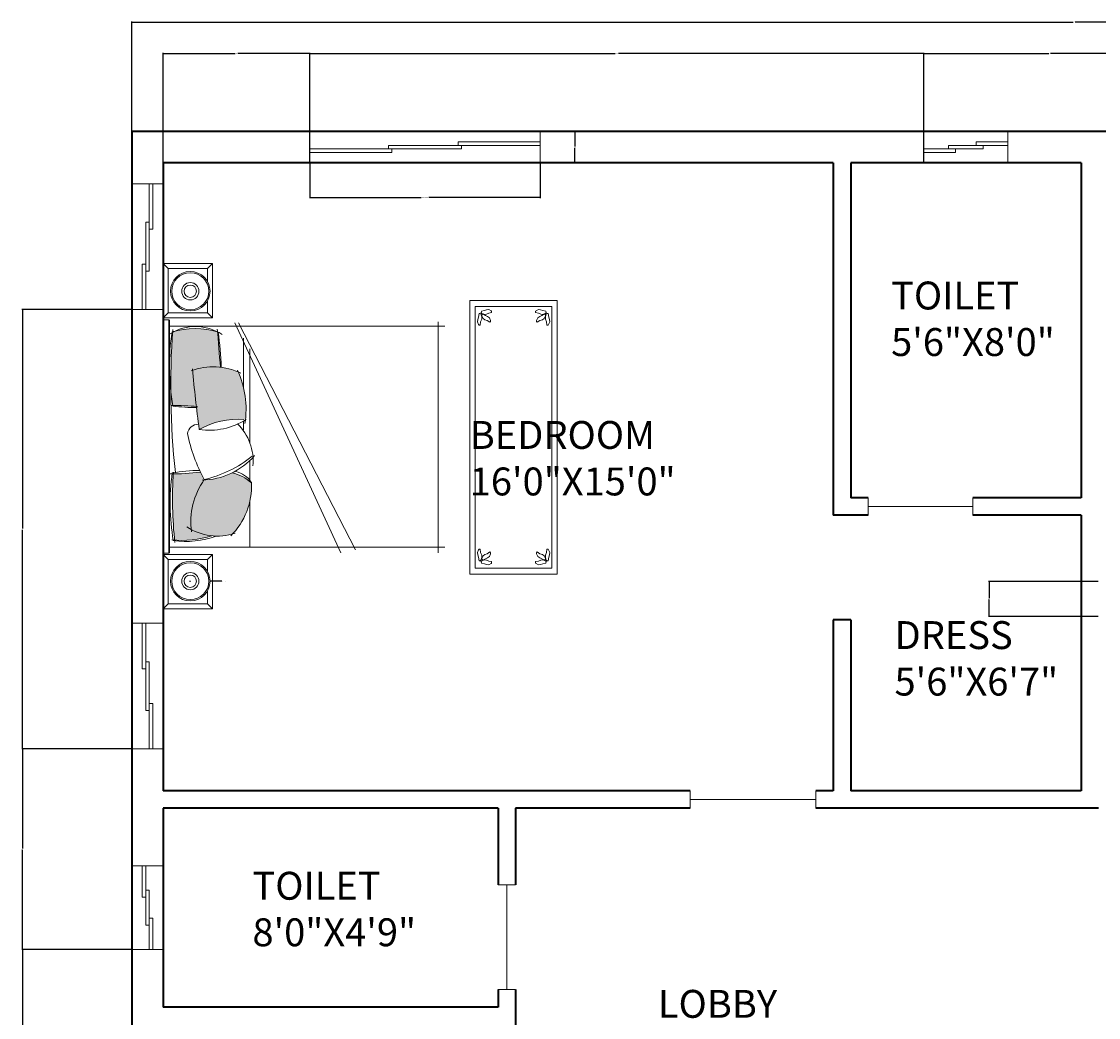
# Model space of a CAD drawing. Units: inches. Extents: x 1569 to 2779, y 1228 to 1844.
# Tile 3 of 6: x 1569 to 1878, y 1559 to 1844. Entities that reach past the tile are written whole.
import ezdxf

# ---------------------------------------------------------------- set-up
doc = ezdxf.new("R2010")
doc.units = ezdxf.units.IN
for name, color, linetype, lineweight in [('0.10', 252, 'Continuous', 9), ('0.15', 34, 'Continuous', 15), ('A-ANNO-DIMS', 2, 'Continuous', 18), ('A-AREA-IDEN', 7, 'Continuous', 18), ('A-DOOR', 3, 'Continuous', 20), ('A-FURN', 8, 'Continuous', 13), ('A-FURN-PATT', 116, 'Continuous', 9), ('A-GLAZ', 5, 'Continuous', 18), ('A-WALL', 7, 'Continuous', 35)]:
    doc.layers.add(name, color=color, linetype=linetype, lineweight=lineweight)
doc.styles.get("Standard").update_dxf_attribs({"font": 'arial.ttf'})
doc.dimstyles.get("Standard").update_dxf_attribs({"dimtxt": 0.18, "dimasz": 0.18, "dimexe": 0.18, "dimexo": 0.0625, "dimgap": 0.09, "dimtad": 0, "dimtih": 1, "dimtoh": 1, "dimdec": 4, "dimzin": 0, "dimdsep": 46, "dimtxsty": 'Standard', "dimcen": 0.09, "dimadec": 0, "dimazin": 0, "dimtfac": 1, "dimtdec": 4, "dimtofl": 0, "dimtmove": 0, "dimatfit": 3, "dimfxl": 1, "dimtolj": 1, "dimtzin": 0, "dimarcsym": 0})

# ---------------------------------------------------------------- blocks, each defined once
blk = doc.blocks.new('camita')
at = {"layer": '0.10'}
for p, q in [((-0.85, -0.045), (0.85, -0.045)), ((-0.805, -0.045), (-0.805, -2.0485)), ((0.805, -0.045), (0.805, -2.0485)), ((-0.8271, -0.521), (0.8464, -1.2932)), ((-0.8271, -0.5476), (0.8236, -1.3992)), ((-0.7161, -0.585), (-0.3554, -0.585)), ((-0.1136, -0.585), (-0.0485, -0.585)), ((-0.638, -0.63), (0.0434, -0.63)), ((0.1749, -0.63), (0.3179, -0.63)), ((0.4739, -0.63), (0.805, -0.63)), ((-0.8354, -2), (0.8464, -2))]:
    blk.add_line(p, q, dxfattribs=at)
blk.add_lwpolyline([(-0.85, -0.0405), (0.85, -0.0405), (0.85, 0), (-0.85, 0)], close=True, dxfattribs=at)
for centre, radius, start, end in [((-0.4574, -0.2364), 0.3443, 147.50996, 213.83359), ((-0.1997, -0.2266), 0.5864, 163.92635, 197.14087), ((-0.3639, -5.8457), 5.7909, 83.80731, 94.12107), ((-0.5104, -1.7232), 1.6781, 80.12554, 98.66187), ((2.3534, -0.0532), 2.5803, 180.10628, 184.38541), ((-1.5443, -0.2452), 1.3333, 359.93941, 7.55329), ((1.5815, -0.2893), 1.3353, 170.38021, 178.99138), ((-1.4396, -0.0609), 1.7117, 352.92911, 0.39592), ((0.4524, -3.0675), 2.9996, 83.90257, 93.67595), ((0.4863, -1.6286), 1.5781, 80.16015, 98.05996), ((0.0294, -0.1377), 0.7262, 342.58415, 6.00484), ((0.1326, -0.1696), 0.6307, 339.92303, 8.74334), ((-0.0543, -0.3633), 0.4542, 159.30257, 206.50263), ((-1.3301, -9.6748), 9.4985, 82.27078, 84.93989), ((-0.007, -0.258), 0.0828, 100.01798, 179.73597), ((-0.2931, -1.4378), 1.2903, 61.97485, 77.84351), ((0.6265, -0.7518), 0.5508, 82.96906, 124.67388), ((0.3203, -0.3944), 0.4043, 341.45245, 33.45121), ((0.4585, -0.5454), 0.5842, 151.04555, 184.14969), ((-0.5341, -0.3393), 0.4875, 327.26442, 9.0473), ((-0.1986, -0.2742), 0.5159, 310.73945, 359.05759), ((-0.5673, -0.0868), 0.9057, 321.69527, 346.46261), ((-1.8672, -14.986), 14.6323, 84.65974, 85.75157), ((-0.4598, 1.4861), 1.9092, 260.95299, 268.65169), ((-0.2002, 0.064), 0.6673, 244.78094, 279.06058), ((0.179, -0.272), 0.3828, 224.52836, 275.22287), ((0.4384, -0.4834), 0.1898, 193.68485, 236.70352), ((0.5707, -0.4317), 0.3145, 192.93877, 221.96363), ((0.3612, -0.133), 0.5096, 267.25889, 315.29965)]:
    blk.add_arc(centre, radius, start, end, dxfattribs=at)
blk = doc.blocks.new('VELADOR')
at = {"layer": '0.15'}
for p, q in [((-0.2475, 0), (-0.2025, -0.045)), ((0.2475, 0), (0.2025, -0.045)), ((-0.2025, -0.405), (-0.2475, -0.45)), ((0.2475, -0.45), (0.2025, -0.405))]:
    blk.add_line(p, q, dxfattribs=at)
blk.add_lwpolyline([(-0.2475, 0), (-0.2475, -0.45), (0.2475, -0.45), (0.2475, 0)], close=True, dxfattribs=at)
blk.add_lwpolyline([(0.0921, -0.405), (0.2025, -0.405), (0.2025, -0.045), (-0.2025, -0.045), (-0.2025, -0.405), (-0.0818, -0.405)], dxfattribs=at)
for radius in [0.18, 0.1688, 0.0788, 0.0563]:
    blk.add_circle((0.0052, -0.2474), radius, dxfattribs=at)
blk = doc.blocks.new('carpet-7')
at = {"color": 0, "linetype": 'ByBlock'}
for p, q in [((-1.0224, 0), (0, 0)), ((0, 0), (0, -0.54)), ((-1.694, -0.54), (-1.694, 0)), ((-1.694, 0), (-1.0224, 0)), ((-1.658, -0.5076), (-1.658, -0.0324)), ((-1.658, -0.0324), (-0.036, -0.0324)), ((-1.6112, -0.0562), (-1.6124, -0.0637)), ((-1.6124, -0.0637), (-1.6088, -0.068)), ((-1.5896, -0.0518), (-1.6112, -0.0562)), ((-1.5752, -0.0486), (-1.5896, -0.0518)), ((-1.5764, -0.0724), (-1.5608, -0.0659)), ((-1.5608, -0.0464), (-1.5752, -0.0486)), ((-1.544, -0.0529), (-1.5608, -0.0464)), ((-1.5608, -0.0659), (-1.5404, -0.0637)), ((-1.5404, -0.0562), (-1.544, -0.0529)), ((-1.5404, -0.0637), (-1.5404, -0.0562)), ((-0.1512, -0.0562), (-0.1476, -0.0529)), ((-0.1512, -0.0637), (-0.1512, -0.0562)), ((-0.1308, -0.0659), (-0.1512, -0.0637)), ((-0.1476, -0.0529), (-0.1308, -0.0464)), ((-0.1308, -0.0464), (-0.1164, -0.0486)), ((-0.1152, -0.0724), (-0.1308, -0.0659)), ((-0.1164, -0.0486), (-0.102, -0.0518)), ((-0.102, -0.0518), (-0.0804, -0.0562)), ((-0.0792, -0.0637), (-0.0828, -0.068)), ((-0.0804, -0.0562), (-0.0792, -0.0637)), ((-0.036, -0.0324), (-0.036, -0.5076)), ((-1.6364, -0.1156), (-1.634, -0.1026)), ((-1.6292, -0.1307), (-1.6364, -0.1156)), ((-1.634, -0.1026), (-1.6304, -0.0896)), ((-1.6304, -0.0896), (-1.6256, -0.0702)), ((-1.6256, -0.1339), (-1.6292, -0.1307)), ((-1.6256, -0.0702), (-1.6172, -0.0691)), ((-1.6172, -0.0691), (-1.6124, -0.0724)), ((-1.6148, -0.1156), (-1.6172, -0.1339)), ((-1.6076, -0.1015), (-1.6148, -0.1156)), ((-1.6124, -0.0724), (-1.6064, -0.0886)), ((-1.6088, -0.068), (-1.5908, -0.0734)), ((-1.6088, -0.0788), (-1.6028, -0.0724)), ((-1.5992, -0.0961), (-1.6088, -0.0788)), ((-1.6064, -0.0886), (-1.6076, -0.1015)), ((-1.6028, -0.0724), (-1.5968, -0.0724)), ((-1.5932, -0.108), (-1.5992, -0.0961)), ((-1.5968, -0.0724), (-1.5812, -0.081)), ((-1.5848, -0.1199), (-1.5932, -0.108)), ((-1.5908, -0.0734), (-1.5764, -0.0724)), ((-1.5692, -0.1274), (-1.5848, -0.1199)), ((-1.5812, -0.081), (-1.5728, -0.0918)), ((-1.5728, -0.0918), (-1.568, -0.1069)), ((-1.5632, -0.1274), (-1.5692, -0.1274)), ((-1.568, -0.1069), (-1.5572, -0.1231)), ((-1.5572, -0.1231), (-1.5632, -0.1274)), ((-0.1236, -0.1069), (-0.1344, -0.1231)), ((-0.1344, -0.1231), (-0.1284, -0.1274)), ((-0.1284, -0.1274), (-0.1224, -0.1274)), ((-0.1188, -0.0918), (-0.1236, -0.1069)), ((-0.1224, -0.1274), (-0.1068, -0.1199)), ((-0.1104, -0.081), (-0.1188, -0.0918)), ((-0.1008, -0.0734), (-0.1152, -0.0724)), ((-0.0948, -0.0724), (-0.1104, -0.081)), ((-0.1068, -0.1199), (-0.0984, -0.108)), ((-0.0828, -0.068), (-0.1008, -0.0734)), ((-0.0984, -0.108), (-0.0924, -0.0961)), ((-0.0888, -0.0724), (-0.0948, -0.0724)), ((-0.0924, -0.0961), (-0.0828, -0.0788)), ((-0.0828, -0.0788), (-0.0888, -0.0724)), ((-0.0792, -0.0724), (-0.0852, -0.0886)), ((-0.0852, -0.0886), (-0.084, -0.1015)), ((-0.084, -0.1015), (-0.0768, -0.1156)), ((-0.0744, -0.0691), (-0.0792, -0.0724)), ((-0.0768, -0.1156), (-0.0744, -0.1339)), ((-0.066, -0.0702), (-0.0744, -0.0691)), ((-0.0612, -0.0896), (-0.066, -0.0702)), ((-0.066, -0.1339), (-0.0624, -0.1307)), ((-0.0624, -0.1307), (-0.0552, -0.1156)), ((-0.0576, -0.1026), (-0.0612, -0.0896)), ((-0.0552, -0.1156), (-0.0576, -0.1026)), ((-1.6172, -0.1339), (-1.6256, -0.1339)), ((-0.0744, -0.1339), (-0.066, -0.1339)), ((-1.6292, -0.4093), (-1.6364, -0.4244)), ((-1.6364, -0.4244), (-1.634, -0.4374)), ((-1.634, -0.4374), (-1.6304, -0.4504)), ((-1.6304, -0.4504), (-1.6256, -0.4698)), ((-1.6256, -0.4061), (-1.6292, -0.4093)), ((-1.6172, -0.4061), (-1.6256, -0.4061)), ((-1.6148, -0.4244), (-1.6172, -0.4061)), ((-1.6076, -0.4385), (-1.6148, -0.4244)), ((-1.6124, -0.4676), (-1.6064, -0.4514)), ((-1.5992, -0.4439), (-1.6088, -0.4612)), ((-1.6088, -0.4612), (-1.6028, -0.4676)), ((-1.6088, -0.472), (-1.5908, -0.4666)), ((-1.6064, -0.4514), (-1.6076, -0.4385)), ((-1.5932, -0.432), (-1.5992, -0.4439)), ((-1.5968, -0.4676), (-1.5812, -0.459)), ((-1.5848, -0.4201), (-1.5932, -0.432)), ((-1.5908, -0.4666), (-1.5764, -0.4676)), ((-1.5692, -0.4126), (-1.5848, -0.4201)), ((-1.5812, -0.459), (-1.5728, -0.4482)), ((-1.5728, -0.4482), (-1.568, -0.4331)), ((-1.5632, -0.4126), (-1.5692, -0.4126)), ((-1.568, -0.4331), (-1.5572, -0.4169)), ((-1.5572, -0.4169), (-1.5632, -0.4126)), ((-0.1344, -0.4169), (-0.1284, -0.4126)), ((-0.1236, -0.4331), (-0.1344, -0.4169)), ((-0.1284, -0.4126), (-0.1224, -0.4126)), ((-0.1188, -0.4482), (-0.1236, -0.4331)), ((-0.1224, -0.4126), (-0.1068, -0.4201)), ((-0.1104, -0.459), (-0.1188, -0.4482)), ((-0.1008, -0.4666), (-0.1152, -0.4676)), ((-0.0948, -0.4676), (-0.1104, -0.459)), ((-0.1068, -0.4201), (-0.0984, -0.432)), ((-0.0828, -0.472), (-0.1008, -0.4666)), ((-0.0984, -0.432), (-0.0924, -0.4439)), ((-0.0924, -0.4439), (-0.0828, -0.4612)), ((-0.0828, -0.4612), (-0.0888, -0.4676)), ((-0.0852, -0.4514), (-0.084, -0.4385)), ((-0.0792, -0.4676), (-0.0852, -0.4514)), ((-0.084, -0.4385), (-0.0768, -0.4244)), ((-0.0768, -0.4244), (-0.0744, -0.4061)), ((-0.0744, -0.4061), (-0.066, -0.4061)), ((-0.066, -0.4061), (-0.0624, -0.4093)), ((-0.0612, -0.4504), (-0.066, -0.4698)), ((-0.0624, -0.4093), (-0.0552, -0.4244)), ((-0.0576, -0.4374), (-0.0612, -0.4504)), ((-0.0552, -0.4244), (-0.0576, -0.4374)), ((-1.658, -0.5076), (-0.036, -0.5076)), ((-1.6256, -0.4698), (-1.6172, -0.4709)), ((-1.6172, -0.4709), (-1.6124, -0.4676)), ((-1.6124, -0.4763), (-1.6088, -0.472)), ((-1.6112, -0.4838), (-1.6124, -0.4763)), ((-1.5896, -0.4882), (-1.6112, -0.4838)), ((-1.6028, -0.4676), (-1.5968, -0.4676)), ((-1.5752, -0.4914), (-1.5896, -0.4882)), ((-1.5764, -0.4676), (-1.5608, -0.4741)), ((-1.5608, -0.4936), (-1.5752, -0.4914)), ((-1.5608, -0.4741), (-1.5404, -0.4763)), ((-1.544, -0.4871), (-1.5608, -0.4936)), ((-1.5404, -0.4838), (-1.544, -0.4871)), ((-1.5404, -0.4763), (-1.5404, -0.4838)), ((-0.1308, -0.4741), (-0.1512, -0.4763)), ((-0.1512, -0.4763), (-0.1512, -0.4838)), ((-0.1512, -0.4838), (-0.1476, -0.4871)), ((-0.1476, -0.4871), (-0.1308, -0.4936)), ((-0.1152, -0.4676), (-0.1308, -0.4741)), ((-0.1308, -0.4936), (-0.1164, -0.4914)), ((-0.1164, -0.4914), (-0.102, -0.4882)), ((-0.102, -0.4882), (-0.0804, -0.4838)), ((-0.0888, -0.4676), (-0.0948, -0.4676)), ((-0.0792, -0.4763), (-0.0828, -0.472)), ((-0.0804, -0.4838), (-0.0792, -0.4763)), ((-0.0744, -0.4709), (-0.0792, -0.4676)), ((-0.066, -0.4698), (-0.0744, -0.4709)), ((0, -0.54), (-1.694, -0.54))]:
    blk.add_line(p, q, dxfattribs=at)
blk = doc.blocks.new('WIN-24IN')
for p, q in [((9, 24), (0, 24)), ((3, 24), (3, 15)), ((4, 24), (4, 7)), ((4, 17), (5, 17)), ((5, 17), (5, 0)), ((3, 15), (4, 15)), ((4, 7), (5, 7)), ((5, 9), (6, 9)), ((6, 9), (6, 0)), ((9, 0), (0, 0))]:
    blk.add_line(p, q)
blk = doc.blocks.new('WIN-66IN')
for p, q in [((0, 0), (0, 9)), ((66, 0), (66, 9)), ((0, 4), (43.5, 4)), ((22.5, 5), (66, 5)), ((22.5, 4), (22.5, 5)), ((23.5, 3), (23.5, 4)), ((42.5, 6), (66, 6)), ((42.5, 5), (42.5, 6)), ((43.5, 4), (43.5, 5)), ((0, 3), (23.5, 3))]:
    blk.add_line(p, q)
blk = doc.blocks.new('WIN-36IN-B')
for p, q in [((0, 36), (9, 36)), ((3, 23), (3, 36)), ((4, 11), (4, 36)), ((5, 25), (4, 25)), ((5, 0), (5, 25)), ((4, 23), (3, 23)), ((6, 13), (5, 13)), ((6, 0), (6, 13)), ((5, 11), (4, 11)), ((0, 0), (9, 0))]:
    blk.add_line(p, q)
blk = doc.blocks.new('DOOR-30IN')
for p, q in [((0, 5), (0, 0)), ((30, 5), (30, 0)), ((0, 2.5), (30, 2.5))]:
    blk.add_line(p, q)
blk = doc.blocks.new('DOOR-36IN')
for p, q in [((0, 5), (0, 0)), ((36, 5), (36, 0)), ((36, 2.5), (0, 2.5))]:
    blk.add_line(p, q)
blk = doc.blocks.new('*D29')
at = {"layer": 'A-ANNO-DIMS', "color": 0, "lineweight": -2, "transparency": 16777216}
for p, q in [((1652.06, 1803.82), (1652.06, 1793.8)), ((1718.06, 1803.82), (1718.06, 1793.8)), ((1652.24, 1793.98), (1683.94, 1793.98)), ((1717.88, 1793.98), (1686.18, 1793.98))]:
    blk.add_line(p, q, dxfattribs=at)
at = {"layer": 'A-ANNO-DIMS', "color": 0, "transparency": 16777216}
for points in [[(1652.24, 1794.01), (1652.24, 1793.95), (1652.06, 1793.98)], [(1717.88, 1794.01), (1717.88, 1793.95), (1718.06, 1793.98)]]:
    blk.add_solid(points, dxfattribs=at)
at = {"layer": 'Defpoints', "color": 0, "transparency": 16777216}
for p in [(1652.06, 1803.88), (1718.06, 1803.88), (1718.06, 1793.98)]:
    blk.add_point(p, dxfattribs=at)
at = {"layer": 'A-ANNO-DIMS', "color": 0, "transparency": 16777216, "insert": (1685.06, 1793.98), "char_height": 0.18, "attachment_point": 5}
blk.add_mtext('\\A1;WINDOW 66 TYP.', dxfattribs=at)
blk = doc.blocks.new('*D30')
at = {"layer": 'A-ANNO-DIMS', "color": 0, "lineweight": -2, "transparency": 16777216}
for p, q in [((1718.12, 1812.88), (1728.14, 1812.88)), ((1727.96, 1812.7), (1727.96, 1808.56)), ((1727.96, 1804.06), (1727.96, 1808.2)), ((1718.12, 1803.88), (1728.14, 1803.88))]:
    blk.add_line(p, q, dxfattribs=at)
at = {"layer": 'A-ANNO-DIMS', "color": 0, "transparency": 16777216}
for points in [[(1727.93, 1812.7), (1727.99, 1812.7), (1727.96, 1812.88)], [(1727.93, 1804.06), (1727.99, 1804.06), (1727.96, 1803.88)]]:
    blk.add_solid(points, dxfattribs=at)
at = {"layer": 'Defpoints', "color": 0, "transparency": 16777216}
for p in [(1718.06, 1812.88), (1727.96, 1812.88), (1718.06, 1803.88)]:
    blk.add_point(p, dxfattribs=at)
at = {"layer": 'A-ANNO-DIMS', "color": 0, "transparency": 16777216, "insert": (1727.96, 1808.38), "char_height": 0.18, "attachment_point": 5}
blk.add_mtext('\\A1;9 TYP.', dxfattribs=at)
blk = doc.blocks.new('*D47')
at = {"layer": 'A-ANNO-DIMS', "color": 0, "lineweight": -2, "transparency": 16777216}
for p, q in [((1601.03, 1812.94), (1601.03, 1844.41)), ((1601.21, 1844.23), (1870.74, 1844.23)), ((2140.85, 1844.23), (1871.32, 1844.23)), ((2141.03, 1812.94), (2141.03, 1844.41))]:
    blk.add_line(p, q, dxfattribs=at)
at = {"layer": 'A-ANNO-DIMS', "color": 0, "transparency": 16777216}
for points in [[(1601.21, 1844.26), (1601.21, 1844.2), (1601.03, 1844.23)], [(2140.85, 1844.26), (2140.85, 1844.2), (2141.03, 1844.23)]]:
    blk.add_solid(points, dxfattribs=at)
at = {"layer": 'Defpoints', "color": 0, "transparency": 16777216}
for p in [(2141.03, 1844.23), (1601.03, 1812.88), (2141.03, 1812.88)]:
    blk.add_point(p, dxfattribs=at)
at = {"layer": 'A-ANNO-DIMS', "color": 0, "transparency": 16777216, "insert": (1871.03, 1844.23), "char_height": 0.18, "attachment_point": 5}
blk.add_mtext('\\A1;540', dxfattribs=at)
blk = doc.blocks.new('*D53')
at = {"layer": 'A-ANNO-DIMS', "color": 0, "lineweight": -2, "transparency": 16777216}
for p, q in [((1610.03, 1803.94), (1610.03, 1835.41)), ((1610.21, 1835.23), (1630.65, 1835.23)), ((1651.88, 1835.23), (1631.44, 1835.23)), ((1652.06, 1803.94), (1652.06, 1835.41))]:
    blk.add_line(p, q, dxfattribs=at)
at = {"layer": 'A-ANNO-DIMS', "color": 0, "transparency": 16777216}
for points in [[(1610.21, 1835.26), (1610.21, 1835.2), (1610.03, 1835.23)], [(1651.88, 1835.26), (1651.88, 1835.2), (1652.06, 1835.23)]]:
    blk.add_solid(points, dxfattribs=at)
at = {"layer": 'Defpoints', "color": 0, "transparency": 16777216}
for p in [(1652.06, 1835.23), (1610.03, 1803.88), (1652.06, 1803.88)]:
    blk.add_point(p, dxfattribs=at)
at = {"layer": 'A-ANNO-DIMS', "color": 0, "transparency": 16777216, "insert": (1631.05, 1835.23), "char_height": 0.18, "attachment_point": 5}
blk.add_mtext('\\A1;42.03', dxfattribs=at)
blk = doc.blocks.new('*D54')
at = {"layer": 'A-ANNO-DIMS', "color": 0, "lineweight": -2, "transparency": 16777216}
for p, q in [((1652.06, 1803.94), (1652.06, 1835.41)), ((1652.24, 1835.23), (1739.59, 1835.23)), ((1827.85, 1835.23), (1740.5, 1835.23)), ((1828.03, 1803.94), (1828.03, 1835.41))]:
    blk.add_line(p, q, dxfattribs=at)
at = {"layer": 'A-ANNO-DIMS', "color": 0, "transparency": 16777216}
for points in [[(1652.24, 1835.26), (1652.24, 1835.2), (1652.06, 1835.23)], [(1827.85, 1835.26), (1827.85, 1835.2), (1828.03, 1835.23)]]:
    blk.add_solid(points, dxfattribs=at)
at = {"layer": 'Defpoints', "color": 0, "transparency": 16777216}
for p in [(1828.03, 1835.23), (1652.06, 1803.88), (1828.03, 1803.88)]:
    blk.add_point(p, dxfattribs=at)
at = {"layer": 'A-ANNO-DIMS', "color": 0, "transparency": 16777216, "insert": (1740.05, 1835.23), "char_height": 0.18, "attachment_point": 5}
blk.add_mtext('\\A1;175.97', dxfattribs=at)
blk = doc.blocks.new('*D55')
at = {"layer": 'A-ANNO-DIMS', "color": 0, "lineweight": -2, "transparency": 16777216}
for p, q in [((1828.03, 1803.94), (1828.03, 1835.41)), ((1828.21, 1835.23), (1863.81, 1835.23)), ((1899.85, 1835.23), (1864.25, 1835.23)), ((1900.03, 1803.94), (1900.03, 1835.41))]:
    blk.add_line(p, q, dxfattribs=at)
at = {"layer": 'A-ANNO-DIMS', "color": 0, "transparency": 16777216}
for points in [[(1828.21, 1835.26), (1828.21, 1835.2), (1828.03, 1835.23)], [(1899.85, 1835.26), (1899.85, 1835.2), (1900.03, 1835.23)]]:
    blk.add_solid(points, dxfattribs=at)
at = {"layer": 'Defpoints', "color": 0, "transparency": 16777216}
for p in [(1900.03, 1835.23), (1828.03, 1803.88), (1900.03, 1803.88)]:
    blk.add_point(p, dxfattribs=at)
at = {"layer": 'A-ANNO-DIMS', "color": 0, "transparency": 16777216, "insert": (1864.03, 1835.23), "char_height": 0.18, "attachment_point": 5}
blk.add_mtext('\\A1;72', dxfattribs=at)
blk = doc.blocks.new('*D63')
at = {"layer": 'A-ANNO-DIMS', "color": 0, "lineweight": -2, "transparency": 16777216}
for p, q in [((1600.97, 1578.38), (1569.5, 1578.38)), ((1569.68, 1578.2), (1569.68, 1547.56)), ((1569.68, 1516.56), (1569.68, 1547.2)), ((1600.97, 1516.38), (1569.5, 1516.38))]:
    blk.add_line(p, q, dxfattribs=at)
at = {"layer": 'A-ANNO-DIMS', "color": 0, "transparency": 16777216}
for points in [[(1569.65, 1578.2), (1569.71, 1578.2), (1569.68, 1578.38)], [(1569.65, 1516.56), (1569.71, 1516.56), (1569.68, 1516.38)]]:
    blk.add_solid(points, dxfattribs=at)
at = {"layer": 'Defpoints', "color": 0, "transparency": 16777216}
for p in [(1569.68, 1578.38), (1601.03, 1578.38), (1601.03, 1516.38)]:
    blk.add_point(p, dxfattribs=at)
at = {"layer": 'A-ANNO-DIMS', "color": 0, "transparency": 16777216, "insert": (1569.68, 1547.38), "char_height": 0.18, "attachment_point": 5}
blk.add_mtext('\\A1;62', dxfattribs=at)
blk = doc.blocks.new('*D64')
at = {"layer": 'A-ANNO-DIMS', "color": 0, "lineweight": -2, "transparency": 16777216}
for p, q in [((1600.97, 1635.88), (1569.5, 1635.88)), ((1569.68, 1635.7), (1569.68, 1607.31)), ((1569.68, 1578.56), (1569.68, 1606.95)), ((1600.97, 1578.38), (1569.5, 1578.38))]:
    blk.add_line(p, q, dxfattribs=at)
at = {"layer": 'A-ANNO-DIMS', "color": 0, "transparency": 16777216}
for points in [[(1569.65, 1635.7), (1569.71, 1635.7), (1569.68, 1635.88)], [(1569.65, 1578.56), (1569.71, 1578.56), (1569.68, 1578.38)]]:
    blk.add_solid(points, dxfattribs=at)
at = {"layer": 'Defpoints', "color": 0, "transparency": 16777216}
for p in [(1569.68, 1635.88), (1601.03, 1635.88), (1601.03, 1578.38)]:
    blk.add_point(p, dxfattribs=at)
at = {"layer": 'A-ANNO-DIMS', "color": 0, "transparency": 16777216, "insert": (1569.68, 1607.13), "char_height": 0.18, "attachment_point": 5}
blk.add_mtext('\\A1;57.5', dxfattribs=at)
blk = doc.blocks.new('*D65')
at = {"layer": 'A-ANNO-DIMS', "color": 0, "lineweight": -2, "transparency": 16777216}
for p, q in [((1600.97, 1761.88), (1569.5, 1761.88)), ((1569.68, 1761.7), (1569.68, 1699.06)), ((1569.68, 1636.06), (1569.68, 1698.7)), ((1600.97, 1635.88), (1569.5, 1635.88))]:
    blk.add_line(p, q, dxfattribs=at)
at = {"layer": 'A-ANNO-DIMS', "color": 0, "transparency": 16777216}
for points in [[(1569.65, 1761.7), (1569.71, 1761.7), (1569.68, 1761.88)], [(1569.65, 1636.06), (1569.71, 1636.06), (1569.68, 1635.88)]]:
    blk.add_solid(points, dxfattribs=at)
at = {"layer": 'Defpoints', "color": 0, "transparency": 16777216}
for p in [(1569.68, 1761.88), (1601.03, 1761.88), (1601.03, 1635.88)]:
    blk.add_point(p, dxfattribs=at)
at = {"layer": 'A-ANNO-DIMS', "color": 0, "transparency": 16777216, "insert": (1569.68, 1698.88), "char_height": 0.18, "attachment_point": 5}
blk.add_mtext('\\A1;126', dxfattribs=at)
blk = doc.blocks.new('*D80')
at = {"layer": 'A-ANNO-DIMS', "color": 0, "lineweight": -2, "transparency": 16777216}
for p, q in [((1877.97, 1683.88), (1846.5, 1683.88)), ((1846.68, 1683.7), (1846.68, 1679.06)), ((1846.68, 1674.06), (1846.68, 1678.7)), ((1877.97, 1673.88), (1846.5, 1673.88))]:
    blk.add_line(p, q, dxfattribs=at)
at = {"layer": 'A-ANNO-DIMS', "color": 0, "transparency": 16777216}
for points in [[(1846.65, 1683.7), (1846.71, 1683.7), (1846.68, 1683.88)], [(1846.65, 1674.06), (1846.71, 1674.06), (1846.68, 1673.88)]]:
    blk.add_solid(points, dxfattribs=at)
at = {"layer": 'Defpoints', "color": 0, "transparency": 16777216}
for p in [(1846.68, 1683.88), (1878.03, 1683.88), (1878.03, 1673.88)]:
    blk.add_point(p, dxfattribs=at)
at = {"layer": 'A-ANNO-DIMS', "color": 0, "transparency": 16777216, "insert": (1846.68, 1678.88), "char_height": 0.18, "attachment_point": 5}
blk.add_mtext('\\A1;10', dxfattribs=at)
blk = doc.blocks.new('*D86')
at = {"layer": 'A-ANNO-DIMS', "color": 0, "lineweight": -2, "transparency": 16777216}
for p, q in [((1617.71, 1683.96), (1617.89, 1683.96)), ((1617.8, 1683.87), (1617.8, 1684.05)), ((1626.85, 1683.96), (1623.64, 1683.96))]:
    blk.add_line(p, q, dxfattribs=at)
at = {"layer": 'A-ANNO-DIMS', "color": 0, "transparency": 16777216}
blk.add_solid([(1623.64, 1683.99), (1623.64, 1683.93), (1623.46, 1683.96)], dxfattribs=at)
at = {"layer": 'Defpoints', "color": 0, "transparency": 16777216}
for p in [(1612.15, 1683.96), (1623.46, 1683.96)]:
    blk.add_point(p, dxfattribs=at)
at = {"layer": 'A-ANNO-DIMS', "color": 0, "transparency": 16777216, "insert": (1627.52, 1683.96), "char_height": 0.18, "attachment_point": 5}
blk.add_mtext('\\A1;2X ∅11.31', dxfattribs=at)

msp = doc.modelspace()

# ---------------------------------------------------------------- hatches: boundary and pattern name
at = {"layer": 'A-FURN-PATT'}
h = msp.add_hatch(color=256, dxfattribs=at)
h.dxf.hatch_style = 1
h.paths.add_polyline_path([(1625.6074, 1755.3888, 0.1310475), (1613.7154, 1755.7666, 0.02065708), (1612.7165, 1755.2602, 0.01851025), (1612.1921, 1738.3915, 0.01544243), (1612.7571, 1734.3504, -0.01670092), (1619.5371, 1734.0816, -0.00696723), (1618.4634, 1744.4488, -0.11389129), (1626.46, 1745.3149, -0.00438694)])
h.paths.add_polyline_path([(1612.9189, 1714.7076, 0.04021238), (1613.3023, 1695.7444, 0.09479225), (1623.9792, 1696.9632, -0.09848778), (1618.0375, 1698.7753, -0.17586366), (1621.7988, 1713.0866, -0.01174183), (1620.7275, 1715.2184, -0.02905141)])
h = msp.add_hatch(color=256, dxfattribs=at)
h.dxf.hatch_style = 1
h.paths.add_polyline_path([(1631.5483, 1743.9727, 0.18953567), (1618.4697, 1744.4952, 0.01140771), (1620.3783, 1727.5384, -0.1503613), (1633.618, 1730.3169, 0.13377603)])
h.paths.add_polyline_path([(1618.0438, 1698.8217, 0.1949524), (1629.9358, 1697.541, 0.20255928), (1635.3187, 1712.2024, 0.12732633), (1629.8112, 1715.0635, -0.10404536), (1621.7085, 1712.9922, 0.17383481)])

# ---------------------------------------------------------------- linework, layer by layer
at = {"layer": 'A-WALL'}
for p, q in [((2141.032, 1812.8785), (1601.032, 1812.8785)), ((1601.032, 1812.8785), (1601.032, 1272.8785)), ((1610.032, 1803.8785), (1610.032, 1623.8785)), ((1802.032, 1803.8785), (1610.032, 1803.8785)), ((1802.032, 1803.8785), (1802.032, 1702.8785)), ((1807.032, 1803.8785), (1807.032, 1707.8785)), ((1873.032, 1803.8785), (1807.032, 1803.8785)), ((1873.032, 1803.8785), (1873.032, 1707.8785)), ((1812.032, 1707.8785), (1807.032, 1707.8785)), ((1873.032, 1707.8785), (1842.032, 1707.8785)), ((1812.032, 1702.8785), (1802.032, 1702.8785)), ((1873.032, 1702.8785), (1842.032, 1702.8785)), ((1873.032, 1702.8785), (1873.032, 1623.8785)), ((1807.032, 1672.8785), (1802.032, 1672.8785)), ((1802.032, 1672.8785), (1802.032, 1623.8785)), ((1807.032, 1672.8785), (1807.032, 1623.8785)), ((1761.032, 1623.8785), (1610.032, 1623.8785)), ((1802.032, 1623.8785), (1797.032, 1623.8785)), ((1873.032, 1623.8785), (1807.032, 1623.8785)), ((1610.032, 1618.8785), (1610.032, 1561.8785)), ((1706.032, 1618.8785), (1610.032, 1618.8785)), ((1706.032, 1618.8785), (1706.032, 1596.8785)), ((1711.032, 1618.8785), (1711.032, 1596.8785)), ((1761.032, 1618.8785), (1711.032, 1618.8785)), ((1878.032, 1618.8785), (1797.032, 1618.8785)), ((1706.032, 1566.8785), (1706.032, 1561.8785)), ((1711.032, 1566.8785), (1711.032, 1499.8785)), ((1706.032, 1561.8785), (1610.032, 1561.8785))]:
    msp.add_line(p, q, dxfattribs=at)

# ---------------------------------------------------------------- block references
at = {"layer": 'A-DOOR'}
for p, rotation in [((1842.032, 1707.8785), 180), ((1706.032, 1596.8785), 270.0000000000017)]:
    msp.add_blockref('DOOR-30IN', p, dxfattribs=dict(at, rotation=rotation))
msp.add_blockref('DOOR-36IN', (1761.032, 1618.8785), dxfattribs=at)
at = {"layer": 'A-FURN'}
for name, p, xscale, yscale, zscale, rotation in [('VELADOR', (1610.032, 1767.2493), -31.41542173157097, 31.41542173157097, 31.41542173157097, 90), ('carpet-7', (1697.9482, 1764.3962), 46.2750735389499, 46.2750735389499, 46.2750735389499, 90), ('camita', (1610.032, 1725.418), -39.375, 39.375, 39.375, 90), ('VELADOR', (1610.032, 1683.7999), 31.41542173157097, 31.41542173157097, 31.41542173157097, 90.00000000000011)]:
    msp.add_blockref(name, p, dxfattribs=dict(at, xscale=xscale, yscale=yscale, zscale=zscale, rotation=rotation))
at = {"layer": 'A-GLAZ'}
for name, p in [('WIN-66IN', (1652.06, 1803.8785)), ('WIN-36IN-B', (1601.032, 1635.8785)), ('WIN-24IN', (1601.032, 1578.3785))]:
    msp.add_blockref(name, p, dxfattribs=at)
at = {"layer": 'A-GLAZ', "rotation": 269.9999999999978}
msp.add_blockref('WIN-24IN', (1828.032, 1812.8785), dxfattribs=at)
at = {"layer": 'A-GLAZ', "extrusion": (0, 0, -1), "zscale": -1, "rotation": 180}
msp.add_blockref('WIN-36IN-B', (-1601.032, 1797.8785), dxfattribs=at)

# ---------------------------------------------------------------- texts
at = {"layer": 'A-AREA-IDEN', "char_height": 8, "attachment_point": 1}
for s, width, heights, insert in [('TOILET\\P5\'6"X8\'0"', 47.685709, [0], (1818.6153, 1769.8574)), ('BEDROOM\\P16\'0"X15\'0"', 101.861325, [0], (1697.8659, 1729.8853)), ('DRESS\\P5\'6"X6\'7"', 101.861325, [21.6389], (1819.5893, 1672.503)), ('TOILET\\P8\'0"X4\'9"', 47.685709, [0], (1635.6037, 1600.6382)), ('   LOBBY\\P14\'0"X9\'11"', 101.861325, [21.6444], (1744.451, 1566.78))]:
    msp.add_mtext_dynamic_manual_height_columns(s, width=width, gutter_width=12.5, heights=heights, dxfattribs=dict(at, insert=insert))

# ---------------------------------------------------------------- dimensions: what is measured, and where the dimension line sits
at = {"layer": 'A-ANNO-DIMS'}
for base, p1, p2, override, picture, middle in [((2141.032, 1844.2285), (1601.032, 1812.8785), (2141.032, 1812.8785), {"dimdec": 0, "dimlfac": 1, "dimrnd": 0, "dimzin": 0, "dimdsep": 46, "dimlunit": 2}, '*D47', (1871.032, 1844.2285)), ((1652.06, 1835.2285), (1610.032, 1803.8785), (1652.06, 1803.8785), {"dimdec": 2, "dimlfac": 1, "dimrnd": 0, "dimzin": 0, "dimdsep": 46, "dimlunit": 2}, '*D53', (1631.046, 1835.2285)), ((1900.032, 1835.2285), (1828.032, 1803.8785), (1900.032, 1803.8785), {"dimdec": 0, "dimlfac": 1, "dimrnd": 0, "dimzin": 0, "dimdsep": 46, "dimlunit": 2}, '*D55', (1864.032, 1835.2285))]:
    dim = msp.add_linear_dim(base=base, p1=p1, p2=p2, dimstyle='Standard', override=override, dxfattribs=at)
    dim.commit()
    dim.dimension.update_dxf_attribs({"geometry": picture, "text_midpoint": middle})
for base, p1, p2, angle, override, picture, middle in [((1828.032, 1835.2285), (1652.06, 1803.8785), (1828.032, 1803.8785), 0, {"dimdec": 2, "dimlfac": 1, "dimrnd": 0, "dimzin": 0, "dimdsep": 46, "dimlunit": 2}, '*D54', (1740.046, 1835.2285)), ((1569.682, 1761.8785), (1601.032, 1635.8785), (1601.032, 1761.8785), 90, {"dimdec": 0, "dimlfac": 1, "dimrnd": 0, "dimzin": 0, "dimdsep": 46, "dimlunit": 2}, '*D65', (1569.682, 1698.8785)), ((1846.682, 1683.8785), (1878.032, 1673.8785), (1878.032, 1683.8785), 90, {"dimdec": 0, "dimlfac": 1, "dimrnd": 0, "dimzin": 0, "dimdsep": 46, "dimlunit": 2}, '*D80', (1846.682, 1678.8785)), ((1569.682, 1635.8785), (1601.032, 1578.3785), (1601.032, 1635.8785), 90, {"dimdec": 1, "dimlfac": 1, "dimrnd": 0, "dimzin": 0, "dimdsep": 46, "dimlunit": 2}, '*D64', (1569.682, 1607.1285)), ((1569.682, 1578.3785), (1601.032, 1516.3785), (1601.032, 1578.3785), 90, {"dimdec": 0, "dimlfac": 1, "dimrnd": 0, "dimzin": 0, "dimdsep": 46, "dimlunit": 2}, '*D63', (1569.682, 1547.3785))]:
    dim = msp.add_linear_dim(base=base, p1=p1, p2=p2, angle=angle, dimstyle='Standard', override=override, dxfattribs=at)
    dim.commit()
    dim.dimension.update_dxf_attribs({"geometry": picture, "text_midpoint": middle})
dim = msp.add_linear_dim(base=(1727.96, 1812.8785), p1=(1718.06, 1803.8785), p2=(1718.06, 1812.8785), angle=90, text='<> TYP.', dimstyle='Standard', override={"dimdec": 0, "dimlfac": 1, "dimrnd": 0, "dimzin": 0, "dimdsep": 46, "dimlunit": 2}, dxfattribs=at)
dim.commit()
dim.dimension.update_dxf_attribs({"geometry": '*D30', "text_midpoint": (1727.96, 1808.3785)})
dim = msp.add_linear_dim(base=(1718.06, 1793.9785), p1=(1652.06, 1803.8785), p2=(1718.06, 1803.8785), text='WINDOW <> TYP.', dimstyle='Standard', override={"dimdec": 0, "dimlfac": 1, "dimrnd": 0, "dimzin": 0, "dimdsep": 46, "dimlunit": 2}, dxfattribs=at)
dim.commit()
dim.dimension.update_dxf_attribs({"geometry": '*D29', "text_midpoint": (1685.06, 1793.9785)})
dim = msp.add_diameter_dim_2p(p1=(1612.1496, 1683.9624), p2=(1623.4592, 1683.962), text='2X <>', dimstyle='Standard', override={"dimdec": 2, "dimlfac": 1, "dimrnd": 0, "dimzin": 0, "dimdsep": 46, "dimlunit": 2}, dxfattribs=at)
dim.commit()
dim.dimension.update_dxf_attribs({"geometry": '*D86', "text_midpoint": (1626.852, 1683.9619), "dimtype": 163})

doc.saveas('drawing.dxf')
